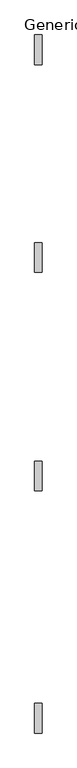
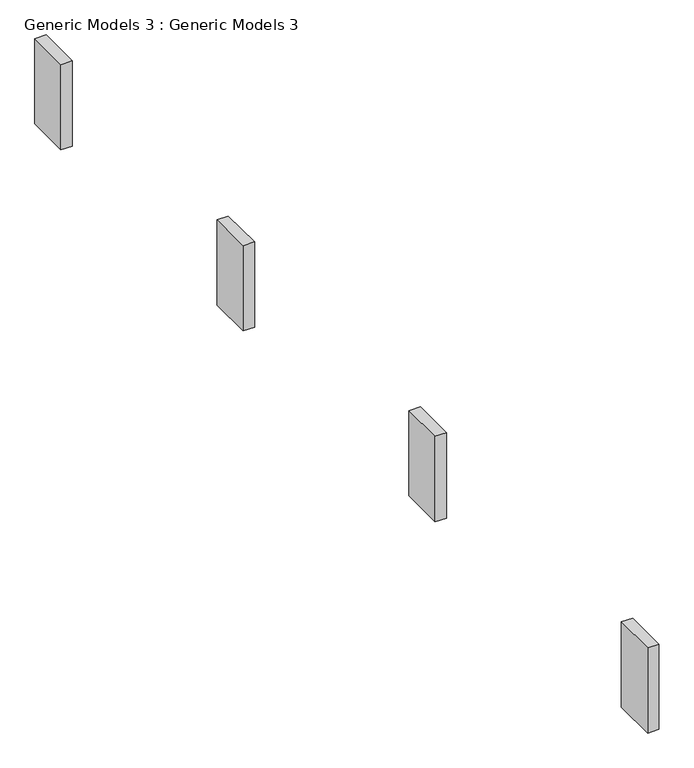
"""IFC4 building model written with IfcOpenShell, lengths in millimetres: proxy geometry, Generic Models 3 : Generic Models 3."""

from ifc_helpers import new_model, si_unit, frame, origin, place, context, project, spatial, polyline, outline, extrude, source, transform, mapped, element, save


def generic_models_3_generic_models_3_96fd7fd6(model_context):
    return source(origin(), model_context, "Body", "SweptSolid", [
        extrude(outline(polyline([(5697.1022658, 7273.4227274), (5697.1022658, 6663.8227274), (5544.7022658, 6663.8227274), (5544.7022658, 7273.4227274), (5697.1022658, 7273.4227274)])), frame((0.0, 0.0, 162.9322), z_axis=(0.0, 0.0, 1.0), x_axis=(1.0, 0.0, 0.0)), (0.0, 0.0, 1.0), 1219.2),
        extrude(outline(polyline([(5697.1022658, 3006.2227274), (5697.1022658, 2396.6227274), (5544.7022658, 2396.6227274), (5544.7022658, 3006.2227274), (5697.1022658, 3006.2227274)])), frame((0.0, 0.0, 162.9322), z_axis=(0.0, 0.0, 1.0), x_axis=(1.0, 0.0, 0.0)), (0.0, 0.0, 1.0), 1219.2),
        extrude(outline(polyline([(5697.1022658, -1489.5772726), (5697.1022658, -2099.1772726), (5544.7022658, -2099.1772726), (5544.7022658, -1489.5772726), (5697.1022658, -1489.5772726)])), frame((0.0, 0.0, 162.9322), z_axis=(0.0, 0.0, 1.0), x_axis=(1.0, 0.0, 0.0)), (0.0, 0.0, 1.0), 1219.2),
        extrude(outline(polyline([(5697.1022658, -6468.0126324), (5697.1022658, -7077.6126324), (5544.7022658, -7077.6126324), (5544.7022658, -6468.0126324), (5697.1022658, -6468.0126324)])), frame((0.0, 0.0, 162.9322), z_axis=(0.0, 0.0, 1.0), x_axis=(1.0, 0.0, 0.0)), (0.0, 0.0, 1.0), 1219.2),
    ])


if __name__ == "__main__":
    model = new_model("IFC4")
    model_context = context("Model", 3, world=origin())
    ifc_project = project(units=[si_unit("LENGTHUNIT", "METRE", prefix="MILLI")], contexts=[model_context])
    site = spatial("IfcSite", under=ifc_project)
    building = spatial("IfcBuilding", under=site)
    placement = place(None, origin())
    generic_models_3_generic_models_3_shape = generic_models_3_generic_models_3_96fd7fd6(model_context)
    element("IfcBuildingElementProxy", 1, Name="Generic Models 3 : Generic Models 3", ObjectType="Generic Models 3 : Generic Models 3", at=placement, inside=building, context=model_context, shape_type="MappedRepresentation", body=[
        mapped(generic_models_3_generic_models_3_shape, transform((0.0, 0.0, 0.0), x_axis=(1.0, 0.0, 0.0), y_axis=(0.0, 1.0, 0.0), z_axis=(0.0, 0.0, 1.0))),
    ])
    save(model, "model.ifc")

# Revit data of these elements
# Element 1 (IfcBuildingElementProxy, "Generic Models 3 : Generic Models 3")
#   Materials on its faces: "legs"
# Materials
#   "legs": colour RGB 90 73 37, transparency 0, Cost = 0
